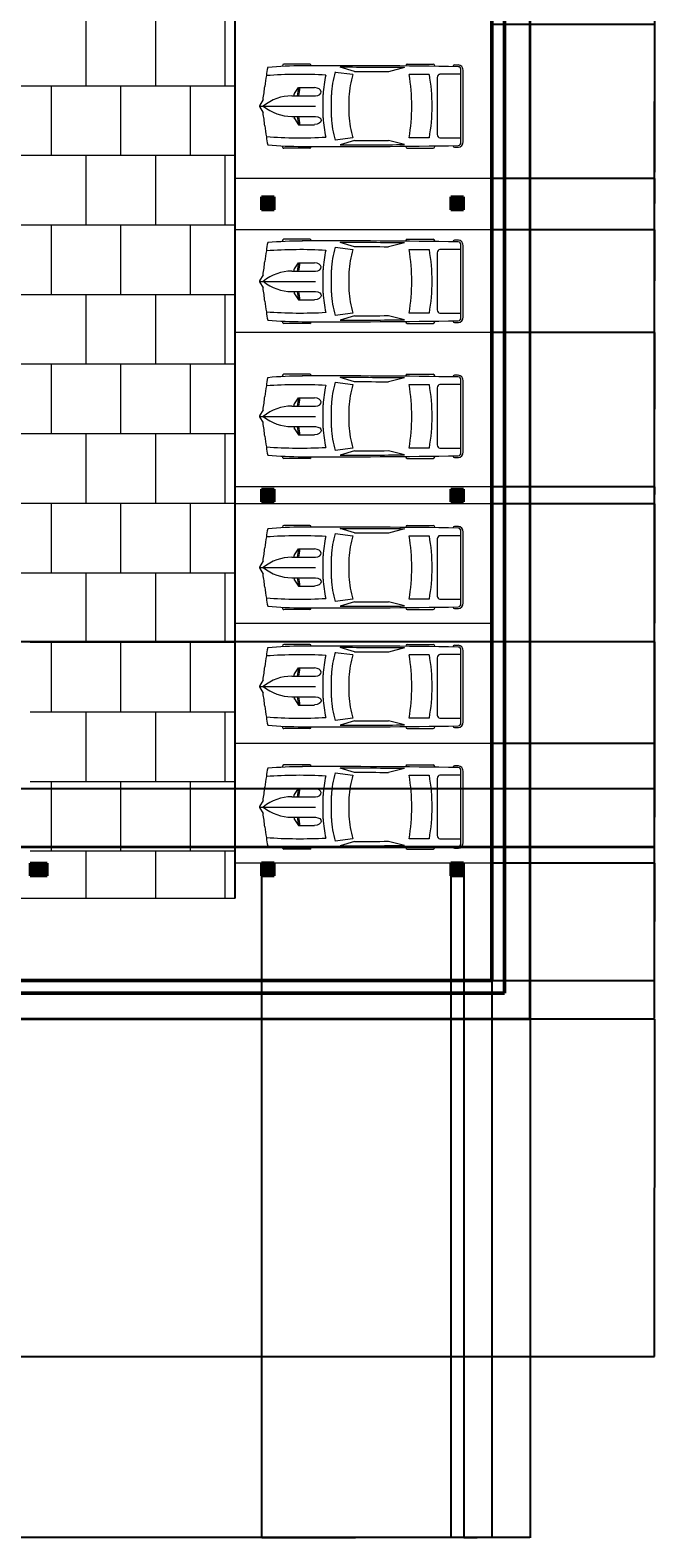
# Model space of a CAD drawing. Units: inches. Extents: x 154617 to 156384, y 250671 to 252576.
# Tile 5 of 6: x 155945 to 156384, y 250671 to 251728. Entities that reach past the tile are written whole.
import ezdxf

# ---------------------------------------------------------------- set-up
doc = ezdxf.new("R2010")
doc.units = ezdxf.units.IN
for name, color, linetype, lineweight in [('A-ANNO-DIMS', 2, 'Continuous', 18), ('A-EQPM-VEHI', 9, 'Continuous', 13), ('A-FLOR-DRIV', 5, 'Continuous', 25), ('A-FLOR-PATT', 112, 'Continuous', 13), ('A-FLOR-PRKG', 4, 'Continuous', 18), ('C-PROP', 5, 'Continuous', 35), ('pillars', 6, 'Continuous', 40), ('walls', 4, 'Continuous', 50)]:
    doc.layers.add(name, color=color, linetype=linetype, lineweight=lineweight)
doc.styles.get("Standard").update_dxf_attribs({"font": 'arial.ttf'})
doc.dimstyles.get("Standard").update_dxf_attribs({"dimtxt": 0.18, "dimasz": 0.18, "dimexe": 0.18, "dimexo": 0.0625, "dimgap": 0.09, "dimtad": 0, "dimtih": 1, "dimtoh": 1, "dimdec": 4, "dimzin": 0, "dimdsep": 46, "dimtxsty": 'Standard', "dimcen": 0.09, "dimadec": 0, "dimazin": 0, "dimtfac": 1, "dimtdec": 4, "dimtofl": 0, "dimtmove": 0, "dimatfit": 3, "dimfxl": 1, "dimtolj": 1, "dimtzin": 0, "dimarcsym": 0})

# ---------------------------------------------------------------- blocks, each defined once
blk = doc.blocks.new('*U2')
for p, q in [((21.1, 37.4), (21.1, 36.8)), ((46.6, 38.9), (22.4, 38.9)), ((47.8, 37.4), (47.8, 37.4)), ((70, 31.5), (86.4, 29.4)), ((88, 31.9), (74.8, 35.9)), ((134.3, 35.6), (119.3, 31.8)), ((135.5, 37.1), (135.5, 37.4)), ((136.7, 38.9), (160.9, 38.9)), ((138.4, 29.4), (157.2, 29.4)), ((162.1, 37.4), (162.1, 36.8)), ((186.5, 29.4), (167, 29.4)), ((186.5, -33.5), (186.5, 33.5)), ((188.4, -32.8), (188.4, 32.8)), ((32.3, 11.6), (36.1, 17.2)), ((36.1, 17.2), (50.9, 17.2)), ((164.5, 26.4), (164.5, -26.4)), ((3.3, 6.1), (0.1, 0.4)), ((29.8, 9.5), (51.7, 9.5)), ((32.1, 9.5), (32.1, 11.2)), ((58.9, -10.8), (58.9, 10.8)), ((66.6, -10.5), (66.6, 10.5)), ((82.7, 8.5), (82.7, -8.5)), ((186.5, -10.5), (186.5, 10.5)), ((0, 0), (51.7, 0)), ((0.1, -0.4), (3.3, -6.1)), ((29.8, -9.5), (51.7, -9.5)), ((32.1, -9.5), (32.1, -11.2)), ((32.3, -11.6), (36.1, -17.2)), ((36.1, -17.2), (50.9, -17.2)), ((21.1, -37.4), (21.1, -36.8)), ((46.6, -38.9), (22.4, -38.9)), ((47.8, -37.4), (47.8, -37.4)), ((86.4, -29.4), (70, -31.5)), ((88, -31.9), (74.8, -35.9)), ((134.3, -35.6), (119.3, -31.8)), ((135.5, -37.1), (135.5, -37.4)), ((136.7, -38.9), (160.9, -38.9)), ((157.2, -29.4), (138.4, -29.4)), ((162.1, -37.4), (162.1, -36.8)), ((167, -29.4), (186.5, -29.4))]:
    blk.add_line(p, q)
for centre, major_axis, ratio, start_param, end_param in [((259.2, -27.5), (0, -305.3), 0.842304, 4.528606, 4.561838), ((266, -27.5), (0, 313.3), 0.842304, 1.367076, 1.39176), ((37.5, -594), (0, -623.3), 0.842304, 3.096046, 3.200911), ((41.2, -490.9), (0, 528.2), 0.842304, 0.00281, 0.075598), ((22.4, 37.4), (0, -1.48), 0.842304, 3.141593, 4.712389), ((64.5, -10555.6), (0, 10593), 0.842304, -0.013397, 0.002797), ((46.6, 37.4), (0, 1.48), 0.842304, -1.570796, 0), ((134.4, 5.4), (0, -89.8), 0.842304, 4.449482, 4.652344), ((135.3, 5.4), (0, 81.8), 0.842304, 1.245306, 1.50788), ((64.5, -10555.6), (0, -10591.5), 0.842304, 3.133765, 3.140441), ((149.6, 2.8), (0, -79.6), 0.842304, 4.372215, 4.640744), ((95.8, -3666.4), (0, -3698.2), 0.842304, 3.134049, 3.144098), ((136.7, 37.4), (0, -1.48), 0.842304, 3.141593, 4.712389), ((17.1, 0), (0, 147), 0.842304, 4.511394, 4.913384), ((35.9, 0), (0, 147), 0.842304, 4.511394, 4.913384), ((160.9, 37.4), (0, 1.48), 0.842304, -1.570796, 0), ((167, 26.4), (0, 2.96), 0.842304, 0, 1.570796), ((180.6, 35.8), (0, 2.22), 0.842304, -0.013017, 1.249894), ((64.5, -10556.4), (0, 10595.3), 0.842304, -0.013397, -0.013017), ((184, 32.8), (0, -5.25), 0.842304, 1.570796, 3.128196), ((184, 33.5), (0, -2.96), 0.842304, 1.570796, 3.128196), ((-204.5, 52.4), (0, -251), 0.842304, 1.385369, 1.434372), ((13, 17), (0, 27.4), 0.842304, 4.435146, 4.718221), ((14.2, 17), (0, 27.4), 0.842304, 4.435146, 4.718221), ((50.8, 13.3), (6.34, -0.36), 0.603834, -1.395552, 1.581315), ((0.6, 0), (0, -0.74), 0.842304, 4.131459, 5.293319), ((29.8, -46.7), (0, 56.2), 0.842304, 0, 0.590319), ((32.7, 11.2), (0, 0.74), 0.842304, 0.879714, 1.570796), ((-204.5, -52.4), (0, 251), 0.842304, -1.434372, -1.385369), ((29.8, 46.7), (0, 56.2), 0.842304, 2.551274, 3.141593), ((32.7, -11.2), (0, -0.74), 0.842304, 4.712389, 5.403472), ((13, -17), (0, -27.4), 0.842304, 1.564964, 1.848039), ((14.2, -17), (0, -27.4), 0.842304, 1.564964, 1.848039), ((134.4, -5.4), (0, -89.8), 0.842304, -1.510751, -1.307889), ((135.3, -5.4), (0, -81.8), 0.842304, -1.50788, -1.245306), ((149.6, -2.8), (0, -79.6), 0.842304, -1.499151, -1.230623), ((259.2, 27.5), (0, 305.3), 0.842304, 1.721348, 1.754579), ((167, -26.4), (0, -2.96), 0.842304, 4.712389, 6.283185), ((266, 27.5), (0, 313.3), 0.842304, 1.749832, 1.774517), ((37.5, 594), (0, -623.3), 0.842304, -0.059319, 0.045547), ((41.2, 490.9), (0, -528.2), 0.842304, -0.075598, -0.00281), ((22.4, -37.4), (0, 1.48), 0.842304, 1.570796, 3.141593), ((64.5, 10555.6), (0, 10593), 0.842304, 3.138796, 3.15499), ((46.6, -37.4), (0, -1.48), 0.842304, 0, 1.570796), ((64.5, 10555.6), (0, -10591.5), 0.842304, 0.001152, 0.007828), ((95.8, 3666.4), (0, -3698.2), 0.842304, -0.002505, 0.007544), ((136.7, -37.4), (0, -1.48), 0.842304, -1.570796, 0), ((160.9, -37.4), (0, 1.48), 0.842304, 3.141593, 4.712389), ((180.6, -35.8), (0, -2.22), 0.842304, -1.249894, 0.013017), ((64.5, 10556.4), (0, 10595.3), 0.842304, 3.15461, 3.15499), ((184, -32.8), (0, -5.25), 0.842304, 0.013397, 1.570796), ((184, -33.5), (0, 2.96), 0.842304, 3.15499, 4.712389)]:
    blk.add_ellipse(centre, major_axis=major_axis, ratio=ratio, start_param=start_param, end_param=end_param)
at = {"extrusion": (0, 0, -1)}
blk.add_ellipse((50.8, -13.3), major_axis=(6.34, 0.36), ratio=0.603834, start_param=-1.395552, end_param=1.581315, dxfattribs=at)
blk = doc.blocks.new('COL-RECT-12x9')
h = blk.add_hatch(color=256)
h.dxf.hatch_style = 1
h.paths.add_polyline_path([(12, 0), (12, 9), (0, 9), (0, 0)])
for p, q in [((12, 9), (0, 9)), ((0, 9), (0, 0)), ((12, 0), (12, 9)), ((0, 0), (12, 0))]:
    blk.add_line(p, q)
blk = doc.blocks.new('COL-RECT-9x9')
h = blk.add_hatch(color=256)
h.dxf.hatch_style = 1
h.paths.add_polyline_path([(0, 9.1), (0, 0), (9, 0), (9, 9.1)])
for p, q in [((9, 9.1), (0, 9.1)), ((0, 9.1), (0, 0)), ((0, 0), (9, 0)), ((9, 0), (9, 9.1))]:
    blk.add_line(p, q)
blk = doc.blocks.new('*D19')
at = {"layer": 'A-ANNO-DIMS', "color": 0, "lineweight": -2, "transparency": 16777216}
for p, q in [((155235.1, 251035), (155235.1, 250671.2)), ((156296.1, 251035), (156296.1, 250671.2)), ((155235.3, 250671.4), (155765.3, 250671.4)), ((156295.9, 250671.4), (155765.9, 250671.4))]:
    blk.add_line(p, q, dxfattribs=at)
at = {"layer": 'A-ANNO-DIMS', "color": 0, "transparency": 16777216}
for points in [[(155235.3, 250671.4), (155235.3, 250671.3), (155235.1, 250671.4)], [(156295.9, 250671.4), (156295.9, 250671.3), (156296.1, 250671.4)]]:
    blk.add_solid(points, dxfattribs=at)
at = {"layer": 'Defpoints', "color": 0, "transparency": 16777216}
for p in [(155235.1, 251035), (156296.1, 251035), (156296.1, 250671.4)]:
    blk.add_point(p, dxfattribs=at)
at = {"layer": 'A-ANNO-DIMS', "color": 0, "transparency": 16777216, "insert": (155765.6, 250671.4), "char_height": 0.18, "attachment_point": 5}
blk.add_mtext('\\A1;1061', dxfattribs=at)
blk = doc.blocks.new('*D20')
at = {"layer": 'A-ANNO-DIMS', "color": 0, "lineweight": -2, "transparency": 16777216}
for p, q in [((156296.2, 252221.5), (156383.4, 252221.5)), ((156383.2, 252221.3), (156383.2, 251628.5)), ((156383.2, 251035.2), (156383.2, 251628.1)), ((156296.2, 251035), (156383.4, 251035))]:
    blk.add_line(p, q, dxfattribs=at)
at = {"layer": 'A-ANNO-DIMS', "color": 0, "transparency": 16777216}
for points in [[(156383.2, 252221.3), (156383.2, 252221.3), (156383.2, 252221.5)], [(156383.2, 251035.2), (156383.2, 251035.2), (156383.2, 251035)]]:
    blk.add_solid(points, dxfattribs=at)
at = {"layer": 'Defpoints', "color": 0, "transparency": 16777216}
for p in [(156296.1, 252221.5), (156383.2, 252221.5), (156296.1, 251035)]:
    blk.add_point(p, dxfattribs=at)
at = {"layer": 'A-ANNO-DIMS', "color": 0, "transparency": 16777216, "insert": (156383.2, 251628.3), "char_height": 0.18, "attachment_point": 5}
blk.add_mtext('\\A1;1186.5', dxfattribs=at)
blk = doc.blocks.new('*D24')
at = {"layer": 'A-ANNO-DIMS', "color": 0, "lineweight": -2, "transparency": 16777216}
for p, q in [((156296.2, 251035), (156383.4, 251035)), ((156383.2, 251034.8), (156383.2, 250916.8)), ((156383.2, 250798.4), (156383.2, 250916.5)), ((155209.3, 250798.3), (156383.4, 250798.3))]:
    blk.add_line(p, q, dxfattribs=at)
at = {"layer": 'A-ANNO-DIMS', "color": 0, "transparency": 16777216}
for points in [[(156383.2, 251034.8), (156383.2, 251034.8), (156383.2, 251035)], [(156383.2, 250798.4), (156383.2, 250798.4), (156383.2, 250798.3)]]:
    blk.add_solid(points, dxfattribs=at)
at = {"layer": 'Defpoints', "color": 0, "transparency": 16777216}
for p in [(156296.1, 251035), (156383.2, 251035), (155209.2, 250798.3)]:
    blk.add_point(p, dxfattribs=at)
at = {"layer": 'A-ANNO-DIMS', "color": 0, "transparency": 16777216, "insert": (156383.2, 250916.6), "char_height": 0.18, "attachment_point": 5}
blk.add_mtext('\\A1;236.76', dxfattribs=at)
blk = doc.blocks.new('*D44')
at = {"layer": 'A-ANNO-DIMS', "color": 0, "lineweight": -2, "transparency": 16777216}
for p, q in [((156269.2, 251732.3), (156383.4, 251732.3)), ((156383.2, 251732.1), (156383.2, 251678.5)), ((156383.2, 251624.5), (156383.2, 251678.1)), ((156269.2, 251624.3), (156383.4, 251624.3))]:
    blk.add_line(p, q, dxfattribs=at)
at = {"layer": 'A-ANNO-DIMS', "color": 0, "transparency": 16777216}
for points in [[(156383.2, 251732.1), (156383.2, 251732.1), (156383.2, 251732.3)], [(156383.2, 251624.5), (156383.2, 251624.5), (156383.2, 251624.3)]]:
    blk.add_solid(points, dxfattribs=at)
at = {"layer": 'Defpoints', "color": 0, "transparency": 16777216}
for p in [(156269.1, 251732.3), (156383.2, 251732.3), (156269.1, 251624.3)]:
    blk.add_point(p, dxfattribs=at)
at = {"layer": 'A-ANNO-DIMS', "color": 0, "transparency": 16777216, "insert": (156383.2, 251678.3), "char_height": 0.18, "attachment_point": 5}
blk.add_mtext('\\A1;108', dxfattribs=at)
blk = doc.blocks.new('*D45')
at = {"layer": 'A-ANNO-DIMS', "color": 0, "lineweight": -2, "transparency": 16777216}
for p, q in [((156269.2, 251624.3), (156383.4, 251624.3)), ((156383.2, 251624.1), (156383.2, 251606.5)), ((156383.2, 251588.5), (156383.2, 251606.1)), ((156269.2, 251588.3), (156383.4, 251588.3))]:
    blk.add_line(p, q, dxfattribs=at)
at = {"layer": 'A-ANNO-DIMS', "color": 0, "transparency": 16777216}
for points in [[(156383.2, 251624.1), (156383.2, 251624.1), (156383.2, 251624.3)], [(156383.2, 251588.5), (156383.2, 251588.5), (156383.2, 251588.3)]]:
    blk.add_solid(points, dxfattribs=at)
at = {"layer": 'Defpoints', "color": 0, "transparency": 16777216}
for p in [(156269.1, 251624.3), (156383.2, 251624.3), (156269.1, 251588.3)]:
    blk.add_point(p, dxfattribs=at)
at = {"layer": 'A-ANNO-DIMS', "color": 0, "transparency": 16777216, "insert": (156383.2, 251606.3), "char_height": 0.18, "attachment_point": 5}
blk.add_mtext('\\A1;36', dxfattribs=at)
blk = doc.blocks.new('*D46')
at = {"layer": 'A-ANNO-DIMS', "color": 0, "lineweight": -2, "transparency": 16777216}
for p, q in [((156269.2, 251588.3), (156383.4, 251588.3)), ((156383.2, 251588.1), (156383.2, 251552.5)), ((156383.2, 251516.5), (156383.2, 251552.1)), ((156269.2, 251516.3), (156383.4, 251516.3))]:
    blk.add_line(p, q, dxfattribs=at)
at = {"layer": 'A-ANNO-DIMS', "color": 0, "transparency": 16777216}
for points in [[(156383.2, 251588.1), (156383.2, 251588.1), (156383.2, 251588.3)], [(156383.2, 251516.5), (156383.2, 251516.5), (156383.2, 251516.3)]]:
    blk.add_solid(points, dxfattribs=at)
at = {"layer": 'Defpoints', "color": 0, "transparency": 16777216}
for p in [(156269.1, 251588.3), (156383.2, 251588.3), (156269.1, 251516.3)]:
    blk.add_point(p, dxfattribs=at)
at = {"layer": 'A-ANNO-DIMS', "color": 0, "transparency": 16777216, "insert": (156383.2, 251552.3), "char_height": 0.18, "attachment_point": 5}
blk.add_mtext('\\A1;72', dxfattribs=at)
blk = doc.blocks.new('*D47')
at = {"layer": 'A-ANNO-DIMS', "color": 0, "lineweight": -2, "transparency": 16777216}
for p, q in [((156269.2, 251516.3), (156383.4, 251516.3)), ((156383.2, 251516.1), (156383.2, 251462.5)), ((156383.2, 251408.5), (156383.2, 251462.1)), ((156269.2, 251408.3), (156383.4, 251408.3))]:
    blk.add_line(p, q, dxfattribs=at)
at = {"layer": 'A-ANNO-DIMS', "color": 0, "transparency": 16777216}
for points in [[(156383.2, 251516.1), (156383.2, 251516.1), (156383.2, 251516.3)], [(156383.2, 251408.5), (156383.2, 251408.5), (156383.2, 251408.3)]]:
    blk.add_solid(points, dxfattribs=at)
at = {"layer": 'Defpoints', "color": 0, "transparency": 16777216}
for p in [(156269.1, 251516.3), (156383.2, 251516.3), (156269.1, 251408.3)]:
    blk.add_point(p, dxfattribs=at)
at = {"layer": 'A-ANNO-DIMS', "color": 0, "transparency": 16777216, "insert": (156383.2, 251462.3), "char_height": 0.18, "attachment_point": 5}
blk.add_mtext('\\A1;108', dxfattribs=at)
blk = doc.blocks.new('*D48')
at = {"layer": 'A-ANNO-DIMS', "color": 0, "lineweight": -2, "transparency": 16777216}
for p, q in [((156269.2, 251408.3), (156383.4, 251408.3)), ((156383.2, 251408.1), (156383.2, 251402.5)), ((156383.2, 251396.5), (156383.2, 251402.1)), ((156269.2, 251396.3), (156383.4, 251396.3))]:
    blk.add_line(p, q, dxfattribs=at)
at = {"layer": 'A-ANNO-DIMS', "color": 0, "transparency": 16777216}
for points in [[(156383.2, 251408.1), (156383.2, 251408.1), (156383.2, 251408.3)], [(156383.2, 251396.5), (156383.2, 251396.5), (156383.2, 251396.3)]]:
    blk.add_solid(points, dxfattribs=at)
at = {"layer": 'Defpoints', "color": 0, "transparency": 16777216}
for p in [(156269.1, 251408.3), (156383.2, 251408.3), (156269.1, 251396.3)]:
    blk.add_point(p, dxfattribs=at)
at = {"layer": 'A-ANNO-DIMS', "color": 0, "transparency": 16777216, "insert": (156383.2, 251402.3), "char_height": 0.18, "attachment_point": 5}
blk.add_mtext('\\A1;12', dxfattribs=at)
blk = doc.blocks.new('*D49')
at = {"layer": 'A-ANNO-DIMS', "color": 0, "lineweight": -2, "transparency": 16777216}
for p, q in [((156269.2, 251396.3), (156383.4, 251396.3)), ((156383.2, 251396.1), (156383.2, 251312.5)), ((156383.2, 251228.5), (156383.2, 251312.1)), ((156269.2, 251228.3), (156383.4, 251228.3))]:
    blk.add_line(p, q, dxfattribs=at)
at = {"layer": 'A-ANNO-DIMS', "color": 0, "transparency": 16777216}
for points in [[(156383.2, 251396.1), (156383.2, 251396.1), (156383.2, 251396.3)], [(156383.2, 251228.5), (156383.2, 251228.5), (156383.2, 251228.3)]]:
    blk.add_solid(points, dxfattribs=at)
at = {"layer": 'Defpoints', "color": 0, "transparency": 16777216}
for p in [(156269.1, 251396.3), (156383.2, 251396.3), (156269.1, 251228.3)]:
    blk.add_point(p, dxfattribs=at)
at = {"layer": 'A-ANNO-DIMS', "color": 0, "transparency": 16777216, "insert": (156383.2, 251312.3), "char_height": 0.18, "attachment_point": 5}
blk.add_mtext('\\A1;168', dxfattribs=at)
blk = doc.blocks.new('*D50')
at = {"layer": 'A-ANNO-DIMS', "color": 0, "lineweight": -2, "transparency": 16777216}
for p, q in [((156269.2, 251228.3), (156383.4, 251228.3)), ((156383.2, 251228.1), (156383.2, 251186.5)), ((156383.2, 251144.5), (156383.2, 251186.1)), ((156269.2, 251144.3), (156383.4, 251144.3))]:
    blk.add_line(p, q, dxfattribs=at)
at = {"layer": 'A-ANNO-DIMS', "color": 0, "transparency": 16777216}
for points in [[(156383.2, 251228.1), (156383.2, 251228.1), (156383.2, 251228.3)], [(156383.2, 251144.5), (156383.2, 251144.5), (156383.2, 251144.3)]]:
    blk.add_solid(points, dxfattribs=at)
at = {"layer": 'Defpoints', "color": 0, "transparency": 16777216}
for p in [(156269.1, 251228.3), (156383.2, 251228.3), (156269.1, 251144.3)]:
    blk.add_point(p, dxfattribs=at)
at = {"layer": 'A-ANNO-DIMS', "color": 0, "transparency": 16777216, "insert": (156383.2, 251186.3), "char_height": 0.18, "attachment_point": 5}
blk.add_mtext('\\A1;84', dxfattribs=at)
blk = doc.blocks.new('*D51')
at = {"layer": 'A-ANNO-DIMS', "color": 0, "lineweight": -2, "transparency": 16777216}
for p, q in [((156269.2, 251144.3), (156383.4, 251144.3)), ((156383.2, 251144.1), (156383.2, 251103.3)), ((156383.2, 251062.2), (156383.2, 251103)), ((156269.2, 251062), (156383.4, 251062))]:
    blk.add_line(p, q, dxfattribs=at)
at = {"layer": 'A-ANNO-DIMS', "color": 0, "transparency": 16777216}
for points in [[(156383.2, 251144.1), (156383.2, 251144.1), (156383.2, 251144.3)], [(156383.2, 251062.2), (156383.2, 251062.2), (156383.2, 251062)]]:
    blk.add_solid(points, dxfattribs=at)
at = {"layer": 'Defpoints', "color": 0, "transparency": 16777216}
for p in [(156269.1, 251144.3), (156383.2, 251144.3), (156269.1, 251062)]:
    blk.add_point(p, dxfattribs=at)
at = {"layer": 'A-ANNO-DIMS', "color": 0, "transparency": 16777216, "insert": (156383.2, 251103.2), "char_height": 0.18, "attachment_point": 5}
blk.add_mtext('\\A1;82.27', dxfattribs=at)
blk = doc.blocks.new('*D53')
at = {"layer": 'A-ANNO-DIMS', "color": 0, "lineweight": -2, "transparency": 16777216}
for p, q in [((155844.7, 251299.5), (156383.4, 251299.5)), ((156383.2, 251299.3), (156383.2, 251227.7)), ((156383.2, 251155.7), (156383.2, 251227.3)), ((155844.7, 251155.5), (156383.4, 251155.5))]:
    blk.add_line(p, q, dxfattribs=at)
at = {"layer": 'A-ANNO-DIMS', "color": 0, "transparency": 16777216}
for points in [[(156383.2, 251299.3), (156383.2, 251299.3), (156383.2, 251299.5)], [(156383.2, 251155.7), (156383.2, 251155.7), (156383.2, 251155.5)]]:
    blk.add_solid(points, dxfattribs=at)
at = {"layer": 'Defpoints', "color": 0, "transparency": 16777216}
for p in [(155844.6, 251299.5), (156383.2, 251299.5), (155844.6, 251155.5)]:
    blk.add_point(p, dxfattribs=at)
at = {"layer": 'A-ANNO-DIMS', "color": 0, "transparency": 16777216, "insert": (156383.2, 251227.5), "char_height": 0.18, "attachment_point": 5}
blk.add_mtext('\\A1;144', dxfattribs=at)
blk = doc.blocks.new('*D63')
at = {"layer": 'A-ANNO-DIMS', "color": 0, "lineweight": -2, "transparency": 16777216}
for p, q in [((156107.5, 251144.2), (156107.5, 250671.2)), ((156240.4, 251144.2), (156240.4, 250671.2)), ((156107.7, 250671.4), (156173.5, 250671.4)), ((156240.2, 250671.4), (156174.4, 250671.4))]:
    blk.add_line(p, q, dxfattribs=at)
at = {"layer": 'A-ANNO-DIMS', "color": 0, "transparency": 16777216}
for points in [[(156107.7, 250671.4), (156107.7, 250671.3), (156107.5, 250671.4)], [(156240.2, 250671.4), (156240.2, 250671.3), (156240.4, 250671.4)]]:
    blk.add_solid(points, dxfattribs=at)
at = {"layer": 'Defpoints', "color": 0, "transparency": 16777216}
for p in [(156107.5, 251144.3), (156240.4, 251144.3), (156240.4, 250671.4)]:
    blk.add_point(p, dxfattribs=at)
at = {"layer": 'A-ANNO-DIMS', "color": 0, "transparency": 16777216, "insert": (156173.9, 250671.4), "char_height": 0.18, "attachment_point": 5}
blk.add_mtext('\\A1;132.89', dxfattribs=at)
blk = doc.blocks.new('*D64')
at = {"layer": 'A-ANNO-DIMS', "color": 0, "lineweight": -2, "transparency": 16777216}
for p, q in [((156249.4, 251144.2), (156249.4, 250671.2)), ((156269.1, 251144.2), (156269.1, 250671.2)), ((156249.5, 250671.4), (156258.8, 250671.4)), ((156268.9, 250671.4), (156259.6, 250671.4))]:
    blk.add_line(p, q, dxfattribs=at)
at = {"layer": 'A-ANNO-DIMS', "color": 0, "transparency": 16777216}
for points in [[(156249.5, 250671.4), (156249.5, 250671.3), (156249.4, 250671.4)], [(156268.9, 250671.4), (156268.9, 250671.3), (156269.1, 250671.4)]]:
    blk.add_solid(points, dxfattribs=at)
at = {"layer": 'Defpoints', "color": 0, "transparency": 16777216}
for p in [(156249.4, 251144.3), (156269.1, 251144.3), (156269.1, 250671.4)]:
    blk.add_point(p, dxfattribs=at)
at = {"layer": 'A-ANNO-DIMS', "color": 0, "transparency": 16777216, "insert": (156259.2, 250671.4), "char_height": 0.18, "attachment_point": 5}
blk.add_mtext('\\A1;19.74', dxfattribs=at)
blk = doc.blocks.new('*D69')
at = {"layer": 'A-ANNO-DIMS', "color": 0, "lineweight": -2, "transparency": 16777216}
for p, q in [((155765.7, 251196.5), (156383.4, 251196.5)), ((156383.2, 251196.3), (156383.2, 251176.4)), ((156383.2, 251156), (156383.2, 251176)), ((155765.4, 251155.9), (156383.4, 251155.9))]:
    blk.add_line(p, q, dxfattribs=at)
at = {"layer": 'A-ANNO-DIMS', "color": 0, "transparency": 16777216}
for points in [[(156383.2, 251196.3), (156383.2, 251196.3), (156383.2, 251196.5)], [(156383.2, 251156), (156383.2, 251156), (156383.2, 251155.9)]]:
    blk.add_solid(points, dxfattribs=at)
at = {"layer": 'Defpoints', "color": 0, "transparency": 16777216}
for p in [(155765.6, 251196.5), (156383.2, 251196.5), (155765.3, 251155.9)]:
    blk.add_point(p, dxfattribs=at)
at = {"layer": 'A-ANNO-DIMS', "color": 0, "transparency": 16777216, "insert": (156383.2, 251176.2), "char_height": 0.18, "attachment_point": 5}
blk.add_mtext('\\A1;40.67', dxfattribs=at)

msp = doc.modelspace()

# ---------------------------------------------------------------- hatches: boundary and pattern name
at = {"layer": 'A-FLOR-PATT'}
h = msp.add_hatch(dxfattribs=at)
h.set_pattern_fill('AR-B88', color=256, scale=0.24)
h.set_pattern_definition([(0, (0, -2.5), (0, 48.768), []), (90, (0, -2.5), (-24.384, 48.768), [48.768, -48.768])])
h.paths.add_polyline_path([(155324.842, 251443.526), (155324.842, 251299.526), (155945.097, 251299.526), (155945.097, 251119.526), (156089.097, 251119.526), (156089.097, 252132.026), (155921.097, 252132.026), (155921.097, 251872.026), (155324.842, 251872.026), (155324.842, 251728.026), (155921.097, 251728.026), (155921.097, 251443.526)])

# ---------------------------------------------------------------- linework, layer by layer
at = {"layer": 'A-FLOR-DRIV'}
msp.add_line((156089.097, 251119.526), (156089.097, 252142.026), dxfattribs=at)
at = {"layer": 'A-FLOR-PRKG'}
for p, q in [((156089.097, 251624.297), (156269.097, 251624.297)), ((156089.097, 251588.297), (156269.097, 251588.297)), ((156089.097, 251516.297), (156269.097, 251516.297)), ((156089.097, 251408.297), (156269.097, 251408.297)), ((156089.097, 251396.297), (156269.097, 251396.297)), ((156089.097, 251312.297), (156269.097, 251312.297)), ((156089.097, 251228.297), (156269.097, 251228.297)), ((156089.097, 251144.297), (156269.097, 251144.297)), ((155262.097, 251119.526), (156089.097, 251119.526))]:
    msp.add_line(p, q, dxfattribs=at)
at = {"layer": 'C-PROP'}
for p, q in [((156296.097, 251035.026), (156296.097, 252221.526)), ((155235.097, 251035.026), (156296.097, 251035.026))]:
    msp.add_line(p, q, dxfattribs=at)
at = {"layer": 'walls'}
for p, q in [((156278.097, 251053.026), (156278.097, 252203.526)), ((156269.097, 251062.026), (156269.097, 252194.526)), ((155262.097, 251062.026), (156269.097, 251062.026)), ((155253.097, 251053.026), (156278.097, 251053.026))]:
    msp.add_line(p, q, dxfattribs=at)

# ---------------------------------------------------------------- block references
at = {"layer": 'A-EQPM-VEHI', "xscale": 0.7581398915747906, "yscale": 0.7581398915747906, "zscale": 0.7581398915747906}
for p in [(156106.107, 251674.88), (156106.107, 251552.043), (156106.107, 251457.378), (156106.107, 251351.444), (156106.107, 251268.05), (156106.107, 251183.529)]:
    msp.add_blockref('*U2', p, dxfattribs=at)
at = {"layer": 'pillars', "rotation": 180}
for p in [(156116.47, 251611.321), (156249.356, 251611.321), (156116.47, 251406.466), (156249.356, 251406.466), (156116.47, 251144.298), (156249.356, 251144.298)]:
    msp.add_blockref('COL-RECT-9x9', p, dxfattribs=at)
at = {"layer": 'pillars'}
msp.add_blockref('COL-RECT-12x9', (155945.159, 251135.26), dxfattribs=at)

# ---------------------------------------------------------------- dimensions: what is measured, and where the dimension line sits
at = {"layer": 'A-ANNO-DIMS'}
for base, p1, p2, override, picture, middle in [((156383.197, 252221.526), (156296.097, 251035.026), (156296.097, 252221.526), {"dimdec": 1, "dimlfac": 1, "dimrnd": 0, "dimzin": 0, "dimdsep": 46, "dimlunit": 2}, '*D20', (156383.197, 251628.276)), ((156383.197, 251732.297), (156269.097, 251624.297), (156269.097, 251732.297), {"dimdec": 0, "dimlfac": 1, "dimrnd": 0, "dimzin": 0, "dimdsep": 46, "dimlunit": 2}, '*D44', (156383.197, 251678.297)), ((156383.197, 251624.297), (156269.097, 251588.297), (156269.097, 251624.297), {"dimdec": 0, "dimlfac": 1, "dimrnd": 0, "dimzin": 0, "dimdsep": 46, "dimlunit": 2}, '*D45', (156383.197, 251606.297)), ((156383.197, 251588.297), (156269.097, 251516.297), (156269.097, 251588.297), {"dimdec": 0, "dimlfac": 1, "dimrnd": 0, "dimzin": 0, "dimdsep": 46, "dimlunit": 2}, '*D46', (156383.197, 251552.297)), ((156383.197, 251516.297), (156269.097, 251408.297), (156269.097, 251516.297), {"dimdec": 0, "dimlfac": 1, "dimrnd": 0, "dimzin": 0, "dimdsep": 46, "dimlunit": 2}, '*D47', (156383.197, 251462.297)), ((156383.197, 251408.297), (156269.097, 251396.297), (156269.097, 251408.297), {"dimdec": 0, "dimlfac": 1, "dimrnd": 0, "dimzin": 0, "dimdsep": 46, "dimlunit": 2}, '*D48', (156383.197, 251402.297)), ((156383.197, 251396.297), (156269.097, 251228.297), (156269.097, 251396.297), {"dimdec": 0, "dimlfac": 1, "dimrnd": 0, "dimzin": 0, "dimdsep": 46, "dimlunit": 2}, '*D49', (156383.197, 251312.297)), ((156383.197, 251299.526), (155844.597, 251155.526), (155844.597, 251299.526), {"dimdec": 0, "dimlfac": 1, "dimrnd": 0, "dimzin": 0, "dimdsep": 46, "dimlunit": 2}, '*D53', (156383.197, 251227.526)), ((156383.197, 251228.297), (156269.097, 251144.297), (156269.097, 251228.297), {"dimdec": 0, "dimlfac": 1, "dimrnd": 0, "dimzin": 0, "dimdsep": 46, "dimlunit": 2}, '*D50', (156383.197, 251186.297)), ((156383.197, 251196.526), (155765.343, 251155.853), (155765.597, 251196.526), {"dimdec": 2, "dimlfac": 1, "dimrnd": 0, "dimzin": 0, "dimdsep": 46, "dimlunit": 2}, '*D69', (156383.197, 251176.189)), ((156383.197, 251144.297), (156269.097, 251062.026), (156269.097, 251144.297), {"dimdec": 2, "dimlfac": 1, "dimrnd": 0, "dimzin": 0, "dimdsep": 46, "dimlunit": 2}, '*D51', (156383.197, 251103.162)), ((156383.197, 251035.026), (155209.237, 250798.266), (156296.097, 251035.026), {"dimdec": 2, "dimlfac": 1, "dimrnd": 0, "dimzin": 0, "dimdsep": 46, "dimlunit": 2}, '*D24', (156383.197, 250916.646))]:
    dim = msp.add_linear_dim(base=base, p1=p1, p2=p2, angle=90, dimstyle='Standard', override=override, dxfattribs=at)
    dim.commit()
    dim.dimension.update_dxf_attribs({"geometry": picture, "text_midpoint": middle})
for base, p1, p2, override, picture, middle in [((156240.3553, 250671.3791), (156107.4701, 251144.2975), (156240.3553, 251144.2975), {"dimdec": 2, "dimlfac": 1, "dimrnd": 0, "dimzin": 0, "dimdsep": 46, "dimlunit": 2}, '*D63', (156173.9127, 250671.3791)), ((156269.097, 250671.379), (156249.355, 251144.297), (156269.097, 251144.297), {"dimdec": 2, "dimlfac": 1, "dimrnd": 0, "dimzin": 0, "dimdsep": 46, "dimlunit": 2}, '*D64', (156259.226, 250671.379)), ((156296.097, 250671.379), (155235.097, 251035.026), (156296.097, 251035.026), {"dimdec": 0, "dimlfac": 1, "dimrnd": 0, "dimzin": 0, "dimdsep": 46, "dimlunit": 2}, '*D19', (155765.597, 250671.379))]:
    dim = msp.add_linear_dim(base=base, p1=p1, p2=p2, dimstyle='Standard', override=override, dxfattribs=at)
    dim.commit()
    dim.dimension.update_dxf_attribs({"geometry": picture, "text_midpoint": middle})

doc.saveas('drawing.dxf')
